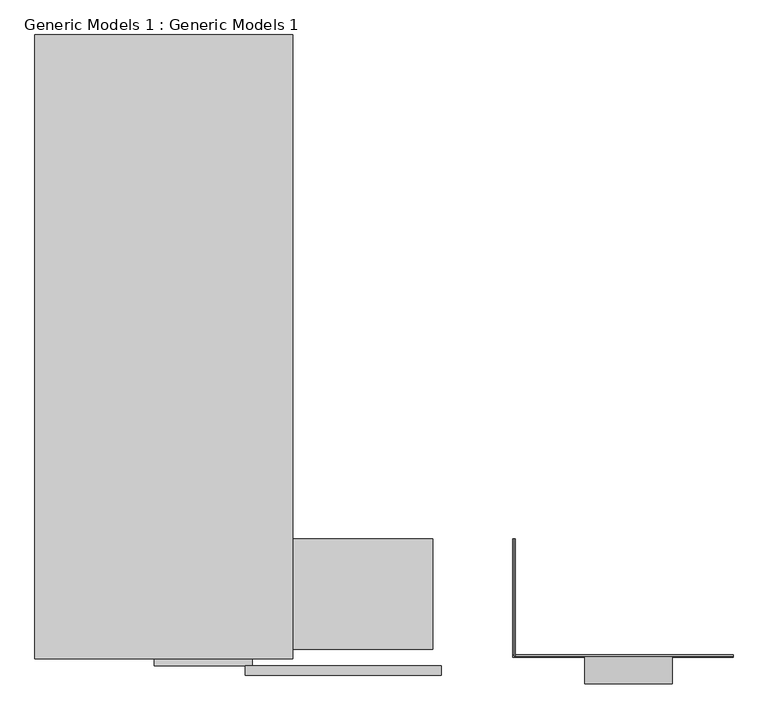
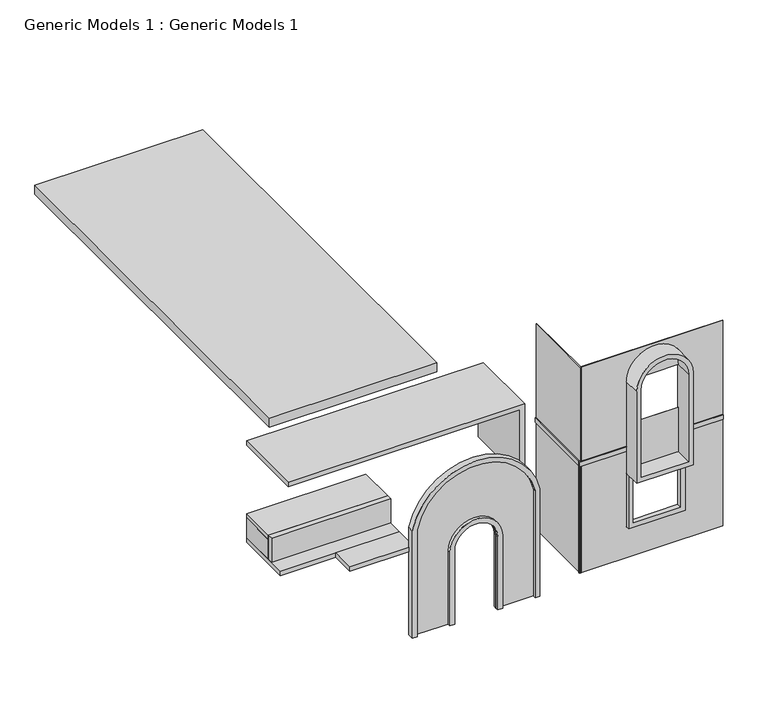
"""IFC4 building model written with IfcOpenShell, lengths in millimetres: proxy geometry, Generic Models 1 : Generic Models 1."""

from ifc_helpers import new_model, si_unit, point, frame, frame_2d, origin, origin_with_axes, place, context, project, spatial, polyline, circle_curve, trimmed, segment, composite_curve, outline, extrude, source, transform, mapped, element, save
from ifc_brep_helpers import plane_surface, cylinder_surface, revolved_surface, advanced_brep


def generic_models_1_generic_models_1_ec26760c(model_context):
    return source(origin(), model_context, "Body", "SolidModel", [
        extrude(outline(polyline([(-7104.6924436, 11297.0765264), (-1694.4924436, 11297.0765264), (-1694.4924436, -1809.3234736), (-7104.6924436, -1809.3234736), (-7104.6924436, 11297.0765264)])), frame((0.0, 0.0, 8533.9641574), z_axis=(0.0, 0.0, 1.0), x_axis=(1.0, 0.0, 0.0)), (0.0, 0.0, 1.0), 304.8),
        extrude(outline(composite_curve([segment(trimmed(circle_curve(frame_2d((6018.3521861, 5360.5135732)), 762.0), [point((6018.3521861, 6122.5135732))], [point((6018.3521861, 4598.5135732))], False, "CARTESIAN"), True, "CONTINUOUS"), segment(polyline([(6018.3521861, 4598.5135732), (6018.3521861, 6122.5135732)]), True, "CONTINUOUS")], self_intersect=False)), frame((0.0, -1771.2234736, 0.0), z_axis=(0.0, 1.0, 0.0), x_axis=(0.0, 0.0, 1.0)), (0.0, 0.0, 1.0), 12.7),
        extrude(outline(polyline([(6122.5135732, -1771.2234736), (4598.5135732, -1771.2234736), (4598.5135732, -1758.5234736), (6122.5135732, -1758.5234736), (6122.5135732, -1771.2234736)])), frame((0.0, 0.0, 3048.0), z_axis=(0.0, 0.0, 1.0), x_axis=(1.0, 0.0, 0.0)), (0.0, 0.0, 1.0), 1509.6208294),
        extrude(outline(polyline([(-6386.9864268, 705.2765264), (-6234.5864268, 705.2765264), (-6234.5864268, -513.9234736), (-6386.9864268, -513.9234736), (-6386.9864268, 705.2765264)])), frame((0.0, 0.0, 2986.014684), z_axis=(0.0, 0.0, 1.0), x_axis=(1.0, 0.0, 0.0)), (0.0, 0.0, 1.0), 671.585316),
        extrude(outline(polyline([(-6386.9864268, -513.9234736), (-2538.8864268, -513.9234736), (-2538.8864268, -688.9469744), (-6386.9864268, -688.9469744), (-6386.9864268, -513.9234736)])), frame((0.0, 0.0, 2986.014684), z_axis=(0.0, 0.0, 1.0), x_axis=(1.0, 0.0, 0.0)), (0.0, 0.0, 1.0), 823.985316),
        extrude(outline(polyline([(-6386.9864268, -513.9234736), (-6386.9864268, 705.2765264), (-2538.8864268, 705.2765264), (-2538.8864268, -513.9234736), (-6386.9864268, -513.9234736)])), frame((0.0, 0.0, 3657.6), z_axis=(0.0, 0.0, 1.0), x_axis=(1.0, 0.0, 0.0)), (0.0, 0.0, 1.0), 152.4),
        extrude(outline(polyline([(6135.6059723, -6386.9864268), (6135.6059723, 1093.3135732), (3810.0, 1093.3135732), (3810.0, 1245.7135732), (6045.2, 1245.7135732), (6288.0059723, 1245.7135732), (6288.0059723, -6386.9864268), (6135.6059723, -6386.9864268)])), frame((0.0, -1618.8234736, 0.0), z_axis=(0.0, 1.0, 0.0), x_axis=(0.0, 0.0, 1.0)), (0.0, 0.0, 1.0), 2324.1),
        extrude(outline(polyline([(2960.2135732, -1758.5234736), (2960.2135732, 705.2765264), (2985.6135732, 705.2765264), (2985.6135732, -1758.5234736), (2960.2135732, -1758.5234736)])), frame((0.0, 0.0, 3810.0), z_axis=(0.0, 0.0, 1.0), x_axis=(1.0, 0.0, 0.0)), (0.0, 0.0, 1.0), 3200.4),
        extrude(outline(composite_curve([segment(polyline([(7010.4, 2985.6135732), (3810.0, 2985.6135732), (3810.0, 4446.1135732), (6018.3521861, 4446.1135732)]), True, "CONTINUOUS"), segment(trimmed(circle_curve(frame_2d((6018.3521861, 5360.5135732)), 914.4), [point((6018.3521861, 4446.1135732))], [point((6018.3521861, 6274.9135732))], True, "CARTESIAN"), True, "CONTINUOUS"), segment(polyline([(6018.3521861, 6274.9135732), (3810.0, 6274.9135732), (3810.0, 7557.6135732), (7010.4, 7557.6135732), (7010.4, 2985.6135732)]), True, "CONTINUOUS")], self_intersect=False)), frame((0.0, -1758.5234736, 0.0), z_axis=(0.0, 1.0, 0.0), x_axis=(0.0, 0.0, 1.0)), (0.0, 0.0, 1.0), 25.4),
        extrude(outline(polyline([(2960.2135732, -1758.5234736), (2960.2135732, 705.2765264), (2985.6135732, 705.2765264), (2985.6135732, -1758.5234736), (2960.2135732, -1758.5234736)])), origin_with_axes(), (0.0, 0.0, 1.0), 3657.6),
        extrude(outline(polyline([(3657.6, 4446.1135732), (3657.6, 2934.8135732), (0.0, 2934.8135732), (0.0, 7557.6135732), (3657.6, 7557.6135732), (3657.6, 6274.9135732), (1066.8, 6274.9135732), (1066.8, 4446.1135732), (3657.6, 4446.1135732)])), frame((0.0, -1758.5234736, 0.0), z_axis=(0.0, 1.0, 0.0), x_axis=(0.0, 0.0, 1.0)), (0.0, 0.0, 1.0), 25.4),
        extrude(outline(polyline([(2934.8135732, -1733.1234736), (2934.8135732, 705.2765264), (2985.6135732, 705.2765264), (2985.6135732, -1733.1234736), (2934.8135732, -1733.1234736)])), frame((0.0, 0.0, 3657.6), z_axis=(0.0, 0.0, 1.0), x_axis=(1.0, 0.0, 0.0)), (0.0, 0.0, 1.0), 152.4),
        extrude(outline(polyline([(4446.1135732, -1783.9234736), (2934.8135732, -1783.9234736), (2934.8135732, -1733.1234736), (4446.1135732, -1733.1234736), (4446.1135732, -1783.9234736)])), frame((0.0, 0.0, 3657.6), z_axis=(0.0, 0.0, 1.0), x_axis=(1.0, 0.0, 0.0)), (0.0, 0.0, 1.0), 152.4),
        extrude(outline(polyline([(7557.6135732, -1783.9234736), (6274.9135732, -1783.9234736), (6274.9135732, -1733.1234736), (7557.6135732, -1733.1234736), (7557.6135732, -1783.9234736)])), frame((0.0, 0.0, 3657.6), z_axis=(0.0, 0.0, 1.0), x_axis=(1.0, 0.0, 0.0)), (0.0, 0.0, 1.0), 152.4),
        extrude(outline(composite_curve([segment(polyline([(2895.6, 6274.9135732), (6018.3521861, 6274.9135732)]), True, "CONTINUOUS"), segment(trimmed(circle_curve(frame_2d((6018.3521861, 5360.5135732)), 914.4), [point((6018.3521861, 6274.9135732))], [point((6018.3521861, 4446.1135732))], False, "CARTESIAN"), True, "CONTINUOUS"), segment(polyline([(6018.3521861, 4446.1135732), (2895.6, 4446.1135732), (2895.6, 6274.9135732)]), True, "CONTINUOUS")], self_intersect=False), holes=[composite_curve([segment(polyline([(3048.0, 4598.5135732), (6018.3521861, 4598.5135732)]), True, "CONTINUOUS"), segment(trimmed(circle_curve(frame_2d((6018.3521861, 5360.5135732)), 762.0), [point((6018.3521861, 4598.5135732))], [point((6018.3521861, 6122.5135732))], True, "CARTESIAN"), True, "CONTINUOUS"), segment(polyline([(6018.3521861, 6122.5135732), (3048.0, 6122.5135732), (3048.0, 4598.5135732)]), True, "CONTINUOUS")], self_intersect=False)]), frame((0.0, -2342.7234736, 0.0), z_axis=(0.0, 1.0, 0.0), x_axis=(0.0, 0.0, 1.0)), (0.0, 0.0, 1.0), 609.6),
        extrude(outline(polyline([(2895.6, 6274.9135732), (2895.6, 4446.1135732), (1066.8, 4446.1135732), (1066.8, 6274.9135732), (2895.6, 6274.9135732)]), holes=[polyline([(2743.2, 6122.5135732), (1219.2, 6122.5135732), (1219.2, 4598.5135732), (2743.2, 4598.5135732), (2743.2, 6122.5135732)])]), frame((0.0, -1885.5234736, 0.0), z_axis=(0.0, 1.0, 0.0), x_axis=(0.0, 0.0, 1.0)), (0.0, 0.0, 1.0), 152.4),
        extrude(outline(composite_curve([segment(polyline([(0.0, 1271.1135732), (3641.7816661, 1271.1135732)]), True, "CONTINUOUS"), segment(trimmed(circle_curve(frame_2d((3234.0872166, -633.8864268)), 1948.1375116), [point((3641.7816661, 1271.1135732))], [point((3641.7816661, -2538.8864268))], False, "CARTESIAN"), True, "CONTINUOUS"), segment(polyline([(3641.7816661, -2538.8864268), (0.0, -2538.8864268), (0.0, -1332.3864268), (2489.2, -1332.3864268)]), True, "CONTINUOUS"), segment(trimmed(circle_curve(frame_2d((2489.2, -633.8864268)), 698.5), [point((2489.2, -1332.3864268))], [point((2489.2, 64.6135732))], True, "CARTESIAN"), True, "CONTINUOUS"), segment(polyline([(2489.2, 64.6135732), (0.0, 64.6135732), (0.0, 1271.1135732)]), True, "CONTINUOUS")], self_intersect=False)), frame((0.0, -2063.3234736, 0.0), z_axis=(0.0, 1.0, 0.0), x_axis=(0.0, 0.0, 1.0)), (0.0, 0.0, 1.0), 101.6),
        advanced_brep(
        [(-1332.3864268, -2164.9234736, 2489.2), (64.6135732, -2164.9234736, 2489.2), (64.6135732, -2164.9234736, 0.0), (217.0135732, -2164.9234736, 0.0), (217.0135732, -2164.9234736, 2489.2), (-1484.7864268, -2164.9234736, 2489.2), (-1484.7864268, -2164.9234736, -1.5875), (-1332.3864268, -2164.9234736, -1.5875), (-1332.3864268, -1961.7234736, -1.5875), (-1484.7864268, -1961.7234736, -1.5875), (-1484.7864268, -1961.7234736, 2489.2), (217.0135732, -1961.7234736, 2489.2), (217.0135732, -1961.7234736, 0.0), (64.6135732, -1961.7234736, 0.0), (64.6135732, -1961.7234736, 2489.2), (-1332.3864268, -1961.7234736, 2489.2), (-1332.3864268, -1961.7234736, 0.0), (-1332.3864268, -2063.3234736, 2489.2), (64.6135732, -2063.3234736, 2489.2), (64.6135732, -2063.3234736, 0.0)],
        [
            (0, 1, circle_curve(frame((-633.8864268, -2164.9234736, 2489.2), z_axis=(0.0, 1.0, 0.0), x_axis=(1.0, 0.0, 0.0)), 698.5)),
            (1, 2),
            (2, 3),
            (3, 4),
            (4, 5, circle_curve(frame((-633.8864268, -2164.9234736, 2489.2), z_axis=(0.0, -1.0, 0.0), x_axis=(1.0, 0.0, 0.0)), 850.9)),
            (5, 6),
            (6, 7),
            (7, 0),
            (8, 9),
            (9, 10),
            (10, 11, circle_curve(frame((-633.8864268, -1961.7234736, 2489.2), z_axis=(0.0, 1.0, 0.0), x_axis=(1.0, 0.0, 0.0)), 850.9)),
            (11, 12),
            (12, 13),
            (13, 14),
            (14, 15, circle_curve(frame((-633.8864268, -1961.7234736, 2489.2), z_axis=(0.0, -1.0, 0.0), x_axis=(1.0, 0.0, 0.0)), 698.5)),
            (15, 16),
            (16, 8),
            (0, 17),
            (17, 15),
            (14, 18),
            (18, 1),
            (13, 19),
            (19, 2),
            (12, 3),
            (11, 4),
            (10, 5),
            (9, 6),
            (8, 7),
        ],
        [
            plane_surface(frame((64.6135732, -2164.9234736, 2489.2), z_axis=(0.0, -1.0, 0.0), x_axis=(0.0, 0.0, -1.0))),
            plane_surface(frame((64.6135732, -1961.7234736, 2489.2), z_axis=(0.0, 1.0, 0.0), x_axis=(0.0, 0.0, 1.0))),
            revolved_surface(polyline([(64.61357320000002, -1961.7234736, 2489.2), (64.61357320000002, -2164.9234736, 2489.2)]), (-633.8864268, -1961.7234736, 2489.2), (0.0, 1.0, 0.0)),
            plane_surface(frame((64.6135732, -2164.9234736, 2489.2), z_axis=(-1.0, 0.0, 0.0), x_axis=(0.0, 1.0, 0.0))),
            plane_surface(frame((64.6135732, -2164.9234736, 0.0), z_axis=(0.0, 0.0, -1.0), x_axis=(0.0, 1.0, 0.0))),
            plane_surface(frame((217.0135732, -2164.9234736, 0.0), z_axis=(1.0, 0.0, 0.0), x_axis=(0.0, 1.0, 0.0))),
            cylinder_surface(frame((-633.8864268, -1961.7234736, 2489.2), z_axis=(0.0, -1.0, 0.0), x_axis=(1.0, 0.0, 0.0)), 850.9),
            plane_surface(frame((-1484.7864268, -2164.9234736, 2489.2), z_axis=(-1.0, 0.0, 0.0), x_axis=(0.0, 1.0, 0.0))),
            plane_surface(frame((-1484.7864268, -2164.9234736, -1.5875), z_axis=(0.0, 0.0, -1.0), x_axis=(0.0, 1.0, 0.0))),
            plane_surface(frame((-1332.3864268, -2164.9234736, -1.5875), z_axis=(1.0, 0.0, 0.0), x_axis=(0.0, 1.0, 0.0))),
        ],
        [
            (0, [[1, 2, 3, 4, 5, 6, 7, 8]]),
            (1, [[9, 10, 11, 12, 13, 14, 15, 16, 17]]),
            (2, [[-1, 18, 19, -15, 20, 21]]),
            (3, [[-2, -21, -20, -14, 22, 23]]),
            (4, [[-3, -23, -22, -13, 24]]),
            (5, [[-4, -24, -12, 25]]),
            (6, [[-5, -25, -11, 26]]),
            (7, [[-6, -26, -10, 27]]),
            (8, [[-7, -27, -9, 28]]),
            (9, [[-8, -28, -17, -16, -19, -18]]),
        ],
    ),
        advanced_brep(
        [(-2691.2864268, -2164.9234736, 3657.6), (-2691.2864268, -2164.9234736, 0.0), (-2538.8864268, -2164.9234736, 0.0), (-2538.8864268, -2164.9234736, 3641.7816661), (1271.1135732, -2164.9234736, 3641.7816661), (1271.1135732, -2164.9234736, 0.0), (1423.5135732, -2164.9234736, 0.0), (1423.5135732, -2164.9234736, 3657.6), (-2691.2864268, -1961.7234736, 3657.6), (1423.5135732, -1961.7234736, 3657.6), (1423.5135732, -1961.7234736, 0.0), (1271.1135732, -1961.7234736, 0.0), (1271.1135732, -1961.7234736, 3641.7816661), (-2538.8864268, -1961.7234736, 3641.7816661), (-2538.8864268, -1961.7234736, 0.0), (-2691.2864268, -1961.7234736, 0.0)],
        [
            (0, 1),
            (1, 2),
            (2, 3),
            (3, 4, circle_curve(frame((-633.8864268, -2164.9234736, 3234.0872166), z_axis=(0.0, 1.0, 0.0), x_axis=(1.0, 0.0, 0.0)), 1948.1375116)),
            (4, 5),
            (5, 6),
            (6, 7),
            (7, 0, circle_curve(frame((-633.8864268, -2164.9234736, 3234.0872166), z_axis=(0.0, -1.0, 0.0), x_axis=(1.0, 0.0, 0.0)), 2100.5375116)),
            (8, 9, circle_curve(frame((-633.8864268, -1961.7234736, 3234.0872166), z_axis=(0.0, 1.0, 0.0), x_axis=(1.0, 0.0, 0.0)), 2100.5375116)),
            (9, 10),
            (10, 11),
            (11, 12),
            (12, 13, circle_curve(frame((-633.8864268, -1961.7234736, 3234.0872166), z_axis=(0.0, -1.0, 0.0), x_axis=(1.0, 0.0, 0.0)), 1948.1375116)),
            (13, 14),
            (14, 15),
            (15, 8),
            (0, 8),
            (15, 1),
            (14, 2),
            (13, 3),
            (12, 4),
            (11, 5),
            (10, 6),
            (9, 7),
        ],
        [
            plane_surface(frame((64.6135732, -2164.9234736, 2489.2), z_axis=(0.0, -1.0, 0.0), x_axis=(0.0, 0.0, -1.0))),
            plane_surface(frame((64.6135732, -1961.7234736, 2489.2), z_axis=(0.0, 1.0, 0.0), x_axis=(0.0, 0.0, 1.0))),
            plane_surface(frame((-2691.2864268, -2164.9234736, 3657.6), z_axis=(-1.0, 0.0, 0.0), x_axis=(0.0, 1.0, 0.0))),
            plane_surface(frame((-2691.2864268, -2164.9234736, 0.0), z_axis=(0.0, 0.0, -1.0), x_axis=(0.0, 1.0, 0.0))),
            plane_surface(frame((-2538.8864268, -2164.9234736, 0.0), z_axis=(1.0, 0.0, 0.0), x_axis=(0.0, 1.0, 0.0))),
            revolved_surface(polyline([(1314.2510848, -1961.7234736, 3234.0872166), (1314.2510848, -2164.9234736, 3234.0872166)]), (-633.8864268, -1961.7234736, 3234.0872166), (0.0, 1.0, 0.0)),
            plane_surface(frame((1271.1135732, -2164.9234736, 3641.7816661), z_axis=(-1.0, 0.0, 0.0), x_axis=(0.0, 1.0, 0.0))),
            plane_surface(frame((1271.1135732, -2164.9234736, 0.0), z_axis=(0.0, 0.0, -1.0), x_axis=(0.0, 1.0, 0.0))),
            plane_surface(frame((1423.5135732, -2164.9234736, 0.0), z_axis=(1.0, 0.0, 0.0), x_axis=(0.0, 1.0, 0.0))),
            cylinder_surface(frame((-633.8864268, -1961.7234736, 3234.0872166), z_axis=(0.0, -1.0, 0.0), x_axis=(1.0, 0.0, 0.0)), 2100.5375116),
        ],
        [
            (0, [[1, 2, 3, 4, 5, 6, 7, 8]]),
            (1, [[9, 10, 11, 12, 13, 14, 15, 16]]),
            (2, [[-1, 17, -16, 18]]),
            (3, [[-2, -18, -15, 19]]),
            (4, [[-3, -19, -14, 20]]),
            (5, [[-4, -20, -13, 21]]),
            (6, [[-5, -21, -12, 22]]),
            (7, [[-6, -22, -11, 23]]),
            (8, [[-7, -23, -10, 24]]),
            (9, [[-8, -24, -9, -17]]),
        ],
    ),
        extrude(outline(polyline([(-2538.8864268, -1961.7234736), (-4596.2864268, -1961.7234736), (-4596.2864268, -1176.6621678), (-2538.8864268, -1176.6621678), (-2538.8864268, -1961.7234736)])), frame((0.0, 0.0, 2833.614684), z_axis=(0.0, 0.0, 1.0), x_axis=(1.0, 0.0, 0.0)), (0.0, 0.0, 1.0), 152.4),
        extrude(outline(polyline([(-2538.8864268, -1176.6621678), (-6386.9864268, -1176.6621678), (-6386.9864268, 705.2765264), (-2538.8864268, 705.2765264), (-2538.8864268, -1176.6621678)])), frame((0.0, 0.0, 2833.614684), z_axis=(0.0, 0.0, 1.0), x_axis=(1.0, 0.0, 0.0)), (0.0, 0.0, 1.0), 152.4),
    ])


if __name__ == "__main__":
    model = new_model("IFC4")
    model_context = context("Model", 3, world=origin())
    ifc_project = project(units=[si_unit("LENGTHUNIT", "METRE", prefix="MILLI")], contexts=[model_context])
    site = spatial("IfcSite", under=ifc_project)
    building = spatial("IfcBuilding", under=site)
    placement = place(None, origin())
    generic_models_1_generic_models_1_shape = generic_models_1_generic_models_1_ec26760c(model_context)
    element("IfcBuildingElementProxy", 1, Name="Generic Models 1 : Generic Models 1", ObjectType="Generic Models 1 : Generic Models 1", at=placement, inside=building, context=model_context, shape_type="MappedRepresentation", body=[
        mapped(generic_models_1_generic_models_1_shape, transform((0.0, 0.0, 0.0), x_axis=(1.0, 0.0, 0.0), y_axis=(0.0, 1.0, 0.0), z_axis=(0.0, 0.0, 1.0))),
    ])
    save(model, "model.ifc")

# Revit data of these elements
# Element 1 (IfcBuildingElementProxy, "Generic Models 1 : Generic Models 1")
#   Materials on its faces: "Gypsum Wall Board", "Laminate, Ivory, Matte", "sky colour", "ash colour"
# Materials
#   "Gypsum Wall Board": class "Generic", colour RGB 127 127 127, transparency 0, Description = "Gypsum Wall Board", Cost = 0
#   "Laminate, Ivory, Matte": class "Plastic", colour RGB 247 247 239, transparency 0, Description = "Plastic Laminate - Ivory, Matte", Cost = 0
#   "sky colour": class "Generic", colour RGB 120 120 120, transparency 0, Cost = 0
#   "ash colour": class "Generic", colour RGB 120 120 120, transparency 0, Cost = 0
